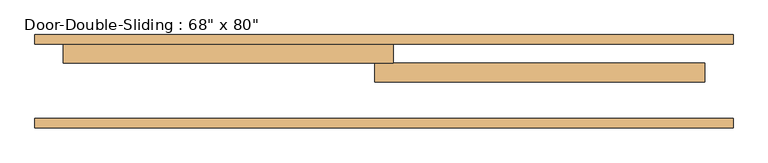
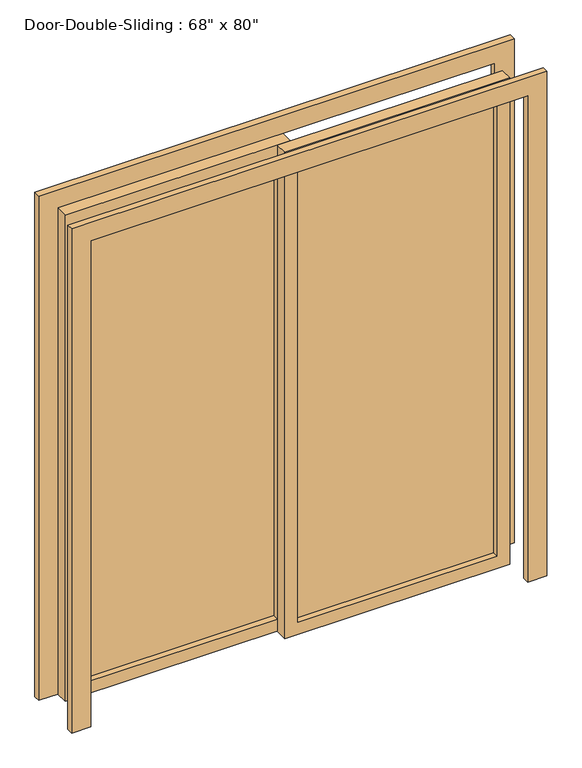
"""IFC4 building model written with IfcOpenShell, lengths in millimetres: door geometry."""

from ifc_helpers import new_model, si_unit, frame, origin, place, context, project, spatial, polyline, outline, extrude, source, transform, mapped, element, save


def door_e30895c2(model_context):
    return source(origin(), model_context, "Body", "SweptSolid", [
        extrude(outline(polyline([(0.0, 939.8), (2108.2, 939.8), (2108.2, -939.8), (0.0, -939.8), (0.0, -863.6), (2032.0, -863.6), (2032.0, 863.6), (0.0, 863.6), (0.0, 939.8)])), frame((0.0, 227.0, 0.0), z_axis=(0.0, 1.0, 0.0), x_axis=(0.0, 0.0, 1.0)), (0.0, 0.0, 1.0), 25.4),
        extrude(outline(polyline([(0.0, -939.8), (0.0, -863.6), (2032.0, -863.6), (2032.0, 863.6), (0.0, 863.6), (0.0, 939.8), (2108.2, 939.8), (2108.2, -939.8), (0.0, -939.8)])), frame((0.0, 1.6, 0.0), z_axis=(0.0, 1.0, 0.0), x_axis=(0.0, 0.0, 1.0)), (0.0, 0.0, 1.0), 25.4),
        extrude(outline(polyline([(2032.0, 25.4), (2032.0, -863.6), (0.0, -863.6), (0.0, 25.4), (2032.0, 25.4)]), holes=[polyline([(1981.2, -25.4), (50.8, -25.4), (50.8, -812.8), (1981.2, -812.8), (1981.2, -25.4)])]), frame((0.0, 176.2, 0.0), z_axis=(0.0, 1.0, 0.0), x_axis=(0.0, 0.0, 1.0)), (0.0, 0.0, 1.0), 50.8),
        extrude(outline(polyline([(2032.0, -25.4), (0.0, -25.4), (0.0, 863.6), (2032.0, 863.6), (2032.0, -25.4)]), holes=[polyline([(1981.2, 25.4), (1981.2, 812.8), (50.8, 812.8), (50.8, 25.4), (1981.2, 25.4)])]), frame((0.0, 125.4, 0.0), z_axis=(0.0, 1.0, 0.0), x_axis=(0.0, 0.0, 1.0)), (0.0, 0.0, 1.0), 50.8),
        extrude(outline(polyline([(-25.4, 200.025), (-812.8, 200.025), (-812.8, 206.375), (-25.4, 206.375), (-25.4, 200.025)])), frame((0.0, 0.0, 50.8), z_axis=(0.0, 0.0, 1.0), x_axis=(1.0, 0.0, 0.0)), (0.0, 0.0, 1.0), 1930.4),
        extrude(outline(polyline([(25.4, 153.975), (812.8, 153.975), (812.8, 147.625), (25.4, 147.625), (25.4, 153.975)])), frame((0.0, 0.0, 50.8), z_axis=(0.0, 0.0, 1.0), x_axis=(1.0, 0.0, 0.0)), (0.0, 0.0, 1.0), 1930.4),
    ])


if __name__ == "__main__":
    model = new_model("IFC4")
    model_context = context("Model", 3, world=origin())
    ifc_project = project(units=[si_unit("LENGTHUNIT", "METRE", prefix="MILLI")], contexts=[model_context])
    site = spatial("IfcSite", under=ifc_project)
    building = spatial("IfcBuilding", under=site)
    placement = place(None, origin())
    door_shape = door_e30895c2(model_context)
    element("IfcDoor", 1, ObjectType="Door-Double-Sliding : 68\" x 80\"", at=placement, inside=building, context=model_context, shape_type="MappedRepresentation", body=[
        mapped(door_shape, transform((0.0, 0.0, 0.0), x_axis=(1.0, 0.0, 0.0), y_axis=(0.0, 1.0, 0.0), z_axis=(0.0, 0.0, 1.0))),
    ])
    save(model, "model.ifc")

# Revit data of these elements
# Type "Door-Double-Sliding : 68\" x 80\""
#   Type Mark = "17"
#   Construction Type Id = "opn-d45"
#   Assembly Code = "C1020"
#   Analytic Construction = "Wood frame, double glass door "
#   Thickness = 0' - 2"
#   Thermal Resistance (R) = 1.8150 (h·ft²·°F)/BTU
#   Heat Transfer Coefficient (U) = 0.5510 BTU/(h·ft²·°F)
#   Height = 6' - 8"
#   Rail Width = 0' - 2"
#   Stiles = 0' - 2"
#   Trim Projection Ext = 0' - 1"
#   Trim Projection Int = 0' - 1"
#   Trim Width = 0' - 3"
#   Width = 5' - 8"
#   Define Thermal Properties by = 1
#   Glazing = Glass
#   Panel Material = Wood - Birch - Solid Stained Light Low Gloss
#   Trim Material = Paint - Sienna
#   Visual Light Transmittance = 0
#   Solar Heat Gain Coefficient = 0
#   Function = (empty or 0)
#   Wall Closure = (empty or 0)
# Element 1 (IfcDoor, "Door-Double-Sliding : 68\" x 80\"")
#   Materials on its faces: "Paint - Sienna", "Wood - Birch - Solid Stained Light Low Gloss", "Glass"
# Materials
#   "Glass": class "Glass", colour RGB 0 128 192, transparency 0.75, Description = "Soda Lime Glass", Cost = 0
#   "Wood - Birch - Solid Stained Light Low Gloss": class "Wood", colour RGB 210 159 95, transparency 0, Cost = 0
#   "Paint - Sienna": colour RGB 118 70 51, transparency 0, Cost = 0
